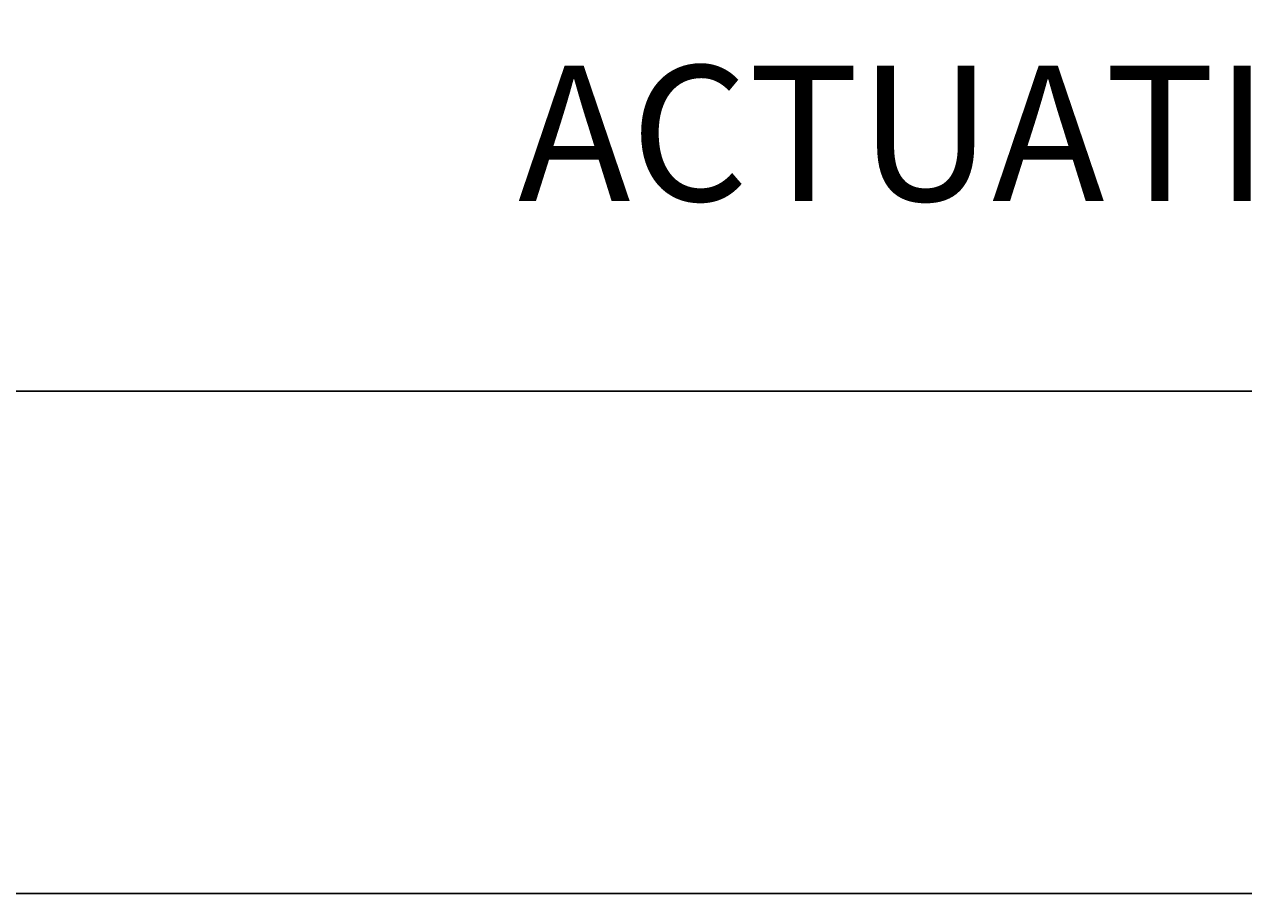
# Model space of a CAD drawing. Units: millimetres. Extents: x -11 to 280, y -4 to 208.
# Tile 25 of 55: x 150 to 186, y -4 to 22. Entities that reach past the tile are written whole.
import ezdxf

# ---------------------------------------------------------------- set-up
doc = ezdxf.new("R2010")
doc.units = ezdxf.units.MM
doc.layers.add('M-ANNO-TEXT', color=7, linetype='Continuous', lineweight=18)
doc.layers.add('M-DIMS', color=2, linetype='Continuous', lineweight=18)
doc.styles.get("Standard").update_dxf_attribs({"font": 'arial.ttf'})
doc.dimstyles.get("Standard").update_dxf_attribs({"dimtxt": 0.18, "dimasz": 0.18, "dimexe": 0.18, "dimexo": 0.0625, "dimgap": 0.09, "dimtad": 0, "dimtih": 1, "dimtoh": 1, "dimdec": 4, "dimzin": 0, "dimdsep": 46, "dimtxsty": 'Standard', "dimcen": 0.09, "dimadec": 0, "dimazin": 0, "dimtfac": 1, "dimtdec": 4, "dimtofl": 0, "dimtmove": 0, "dimatfit": 3, "dimfxl": 1, "dimtolj": 1, "dimtzin": 0, "dimarcsym": 0})

# ---------------------------------------------------------------- blocks, each defined once
blk = doc.blocks.new('*D4')
at = {"layer": 'Defpoints', "color": 0, "transparency": 16777216}
for p in [(4.763, 84.426), (266.035, 51.733), (266.035, -3.415)]:
    blk.add_point(p, dxfattribs=at)
at = {"layer": 'M-DIMS', "color": 0, "lineweight": -2, "transparency": 16777216}
for p, q in [((4.763, 84.364), (4.763, -3.595)), ((266.035, 51.67), (266.035, -3.595)), ((4.943, -3.415), (134.934, -3.415)), ((265.855, -3.415), (135.864, -3.415))]:
    blk.add_line(p, q, dxfattribs=at)
at = {"layer": 'M-DIMS', "color": 0, "transparency": 16777216}
for points in [[(4.943, -3.385), (4.943, -3.445), (4.763, -3.415)], [(265.855, -3.385), (265.855, -3.445), (266.035, -3.415)]]:
    blk.add_solid(points, dxfattribs=at)
at = {"layer": 'M-DIMS', "color": 0, "transparency": 16777216, "insert": (135.399, -3.415), "char_height": 0.18, "attachment_point": 5}
blk.add_mtext('\\A1;261.27', dxfattribs=at)
blk = doc.blocks.new('*D5')
at = {"layer": 'Defpoints', "color": 0, "transparency": 16777216}
for p in [(24.759, 192.645), (-10.087, 11.435), (261.686, 11.435)]:
    blk.add_point(p, dxfattribs=at)
at = {"layer": 'M-DIMS', "color": 0, "lineweight": -2, "transparency": 16777216}
for p, q in [((24.696, 192.645), (-10.267, 192.645)), ((-10.087, 192.465), (-10.087, 102.222)), ((-10.087, 11.615), (-10.087, 101.858)), ((261.624, 11.435), (-10.267, 11.435))]:
    blk.add_line(p, q, dxfattribs=at)
at = {"layer": 'M-DIMS', "color": 0, "transparency": 16777216}
for points in [[(-10.117, 192.465), (-10.057, 192.465), (-10.087, 192.645)], [(-10.117, 11.615), (-10.057, 11.615), (-10.087, 11.435)]]:
    blk.add_solid(points, dxfattribs=at)
at = {"layer": 'M-DIMS', "color": 0, "transparency": 16777216, "insert": (-10.087, 102.04), "char_height": 0.18, "attachment_point": 5}
blk.add_mtext('\\A1;181.2', dxfattribs=at)

msp = doc.modelspace()

# ---------------------------------------------------------------- texts
at = {"layer": 'M-ANNO-TEXT', "insert": (164.865, 21.0543), "char_height": 4, "attachment_point": 1}
msp.add_mtext_dynamic_manual_height_columns('ACTUATING CYLINDER', width=63.617875, gutter_width=12.5, heights=[0], dxfattribs=at)

# ---------------------------------------------------------------- dimensions: what is measured, and where the dimension line sits
at = {"layer": 'M-DIMS'}
dim = msp.add_linear_dim(base=(-10.0865, 11.4346), p1=(24.7588, 192.645), p2=(261.6863, 11.4346), angle=90, dimstyle='Standard', override={"dimdec": 1, "dimlfac": 1, "dimrnd": 0, "dimzin": 0, "dimdsep": 46, "dimlunit": 2}, dxfattribs=at)
dim.commit()
dim.dimension.update_dxf_attribs({"geometry": '*D5', "text_midpoint": (-10.0865, 102.0398)})
dim = msp.add_linear_dim(base=(266.0352, -3.4154), p1=(4.7635, 84.4261), p2=(266.0352, 51.7328), dimstyle='Standard', override={"dimdec": 2, "dimlfac": 1, "dimrnd": 0, "dimzin": 0, "dimdsep": 46, "dimlunit": 2}, dxfattribs=at)
dim.commit()
dim.dimension.update_dxf_attribs({"geometry": '*D4', "text_midpoint": (135.3993, -3.4154)})

doc.saveas('drawing.dxf')
